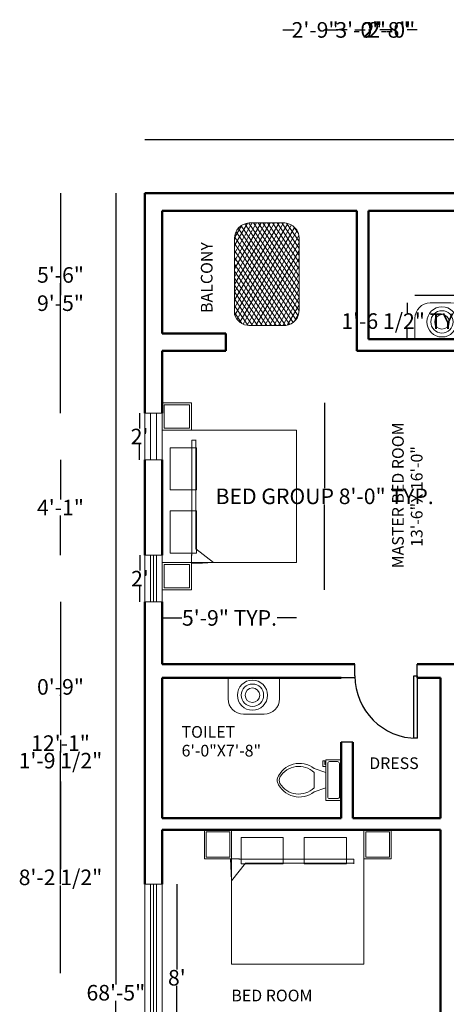
# Model space of a CAD drawing. Units: inches. Extents: x -135167 to -134597, y 156853 to 157819.
# Tile 3 of 5: x -135167 to -134948, y 157306 to 157812. Entities that reach past the tile are written whole.
import ezdxf

# ---------------------------------------------------------------- set-up
doc = ezdxf.new("R2010")
doc.units = ezdxf.units.IN
doc.header["$MEASUREMENT"] = 0
for name, color, linetype, lineweight in [('A-ANNO-DIMS', 4, 'Continuous', 18), ('A-AREA-IDEN', 76, 'Continuous', 25), ('A-FLOR-FIXT', 3, 'Continuous', 20), ('A-FLOR-PATT', 8, 'Continuous', 13), ('A-FURN', 1, 'Continuous', 18), ('doors', 5, 'Continuous', 25), ('walls', 2, 'Continuous', 50), ('window', 6, 'Continuous', 18)]:
    doc.layers.add(name, color=color, linetype=linetype, lineweight=lineweight)
doc.styles.get("Standard").update_dxf_attribs({"font": 'arial.ttf'})
doc.dimstyles.get("Standard").update_dxf_attribs({"dimtxt": 8, "dimasz": 0.18, "dimexe": 0.18, "dimexo": 0.0625, "dimgap": 0.09, "dimtad": 0, "dimtih": 1, "dimtoh": 1, "dimdec": 0, "dimzin": 0, "dimdsep": 46, "dimlunit": 3, "dimtxsty": 'Standard', "dimblk": 'ARCHTICK', "dimcen": 0.09, "dimse1": 1, "dimse2": 1, "dimadec": 0, "dimazin": 0, "dimtfac": 1, "dimtdec": 0, "dimtofl": 0, "dimtmove": 0, "dimatfit": 3, "dimldrblk": 'DOTSMALL', "dimfxl": 1, "dimtolj": 1, "dimtzin": 0, "dimarcsym": 0})

# ---------------------------------------------------------------- blocks, each defined once
blk = doc.blocks.new('*U11')
for p, q in [((-32, 0), (-32, 6)), ((0, 0), (0, 6))]:
    blk.add_line(p, q)
blk.add_lwpolyline([(0, 0), (0, -32), (-1.75, -32), (-1.75, 0)], close=True)
blk.add_arc((0, 0), 32, 180, 270)
blk = doc.blocks.new('*U16')
for p, q in [((-8.01, 3.98), (-14.01, 5.97)), ((-9.51, 6.98), (-9.52, 9.98)), ((-9.52, 9.98), (-8.52, 9.98)), ((-8.01, 6.98), (-9.51, 6.98)), ((-8.52, 9.98), (-8.52, 7.98)), ((-8.52, 7.98), (-8.02, 7.98)), ((-13.99, -4.03), (-14.01, 3.97)), ((-7.99, -4.02), (-13.99, -6.03)), ((-5.98, -9.51), (-1.98, -9.5))]:
    blk.add_line(p, q)
blk.add_lwpolyline([(-7.98, -10.51), (0.02, -10.5), (-0.02, 10.5), (-8.02, 10.48)], close=True)
for points in [[(-7.02, 8.49), (-6.98, -8.51)], [(-2.02, 9.5), (-6.02, 9.49)], [(-0.98, -8.5), (-1.02, 8.5)]]:
    blk.add_lwpolyline(points)
for centre, radius, start, end in [((-21.57, -3.56), 12.17, 51.5766, 158.079), ((-21.81, -4.24), 11.33, 46.4753, 149.0544), ((-6.14, 8.61), 0.884, 81.9774, 188.2376), ((-1.89, 8.62), 0.884, 351.9774, 98.2376), ((-29, -0.05), 4, 164.9681, 195.247), ((-27.88, -0.05), 4, 155.8394, 204.3757), ((-21.59, 3.48), 12.17, 202.136, 308.6382), ((-21.83, 4.16), 11.33, 211.1605, 313.7396), ((-6.11, -8.64), 0.884, 171.9774, 278.2376), ((-1.86, -8.63), 0.884, 261.9774, 8.2376)]:
    blk.add_arc(centre, radius, start, end)
blk = doc.blocks.new('_ArchTick')
at = {"color": 0, "linetype": 'ByBlock', "const_width": 0.15}
blk.add_lwpolyline([(-0.5, -0.5), (0.5, 0.5)], dxfattribs=at)
blk = doc.blocks.new('*D19')
at = {"layer": 'A-ANNO-DIMS', "color": 0, "lineweight": -2, "transparency": 16777216}
for p, q in [((-135102.89, 157750.46), (-134940.89, 157750.46)), ((-134744.89, 157750.46), (-134906.88, 157750.46))]:
    blk.add_line(p, q, dxfattribs=at)
at = {"layer": 'Defpoints', "color": 0, "transparency": 16777216}
for p in [(-134744.89, 157750.46), (-135102.89, 157722.94), (-134744.89, 157722.94)]:
    blk.add_point(p, dxfattribs=at)
at = {"layer": 'A-ANNO-DIMS', "color": 0, "lineweight": -2, "transparency": 16777216, "xscale": 0.18, "yscale": 0.18, "zscale": 0.18, "rotation": 180}
blk.add_blockref('_ArchTick', (-135102.89, 157750.46), dxfattribs=at)
at = {"layer": 'A-ANNO-DIMS', "color": 0, "lineweight": -2, "transparency": 16777216, "xscale": 0.18, "yscale": 0.18, "zscale": 0.18}
blk.add_blockref('_ArchTick', (-134744.89, 157750.46), dxfattribs=at)
at = {"layer": 'A-ANNO-DIMS', "color": 0, "transparency": 16777216, "insert": (-134923.89, 157750.46), "char_height": 8, "attachment_point": 5}
blk.add_mtext('\\A1;29\'-10"', dxfattribs=at)
blk = doc.blocks.new('_DotSmall')
at = {"color": 0, "linetype": 'ByBlock', "const_width": 0.5}
blk.add_lwpolyline([(-0.0625, 0, 1), (0.0625, 0, 1)], format="xyb", close=True, dxfattribs=at)
blk = doc.blocks.new('*D20')
at = {"layer": 'A-ANNO-DIMS', "color": 0, "lineweight": -2, "transparency": 16777216}
for p, q in [((-135117.79, 157722.94), (-135117.79, 157316.42)), ((-135117.79, 156901.55), (-135117.79, 157308.07))]:
    blk.add_line(p, q, dxfattribs=at)
at = {"layer": 'Defpoints', "color": 0, "transparency": 16777216}
for p in [(-135117.79, 157722.94), (-135102.89, 157722.94), (-135102.89, 156901.55)]:
    blk.add_point(p, dxfattribs=at)
at = {"layer": 'A-ANNO-DIMS', "color": 0, "lineweight": -2, "transparency": 16777216, "xscale": 0.18, "yscale": 0.18, "zscale": 0.18}
for p, rotation in [((-135117.79, 157722.94), 90), ((-135117.79, 156901.55), 270)]:
    blk.add_blockref('_ArchTick', p, dxfattribs=dict(at, rotation=rotation))
at = {"layer": 'A-ANNO-DIMS', "color": 0, "transparency": 16777216, "insert": (-135117.79, 157312.25), "char_height": 8, "attachment_point": 5}
blk.add_mtext('\\A1;68\'-5"', dxfattribs=at)
blk = doc.blocks.new('*D31')
at = {"layer": 'A-ANNO-DIMS', "color": 0, "lineweight": -2, "transparency": 16777216}
for p, q in [((-135105.6, 157609.94), (-135105.6, 157602.05)), ((-135105.6, 157585.94), (-135105.6, 157593.84))]:
    blk.add_line(p, q, dxfattribs=at)
at = {"layer": 'Defpoints', "color": 0, "transparency": 16777216}
for p in [(-135102.89, 157609.94), (-135105.6, 157585.94), (-135102.89, 157585.94)]:
    blk.add_point(p, dxfattribs=at)
at = {"layer": 'A-ANNO-DIMS', "color": 0, "lineweight": -2, "transparency": 16777216, "xscale": 0.18, "yscale": 0.18, "zscale": 0.18}
for p, rotation in [((-135105.6, 157609.94), 90), ((-135105.6, 157585.94), 270)]:
    blk.add_blockref('_ArchTick', p, dxfattribs=dict(at, rotation=rotation))
at = {"layer": 'A-ANNO-DIMS', "color": 0, "transparency": 16777216, "insert": (-135105.6, 157597.94), "char_height": 8, "attachment_point": 5}
blk.add_mtext("\\A1;2'", dxfattribs=at)
blk = doc.blocks.new('*D32')
at = {"layer": 'A-ANNO-DIMS', "color": 0, "lineweight": -2, "transparency": 16777216}
for p, q in [((-135105.42, 157536.94), (-135105.42, 157529.05)), ((-135105.42, 157512.94), (-135105.42, 157520.84))]:
    blk.add_line(p, q, dxfattribs=at)
at = {"layer": 'Defpoints', "color": 0, "transparency": 16777216}
for p in [(-135102.89, 157536.94), (-135105.42, 157512.94), (-135102.89, 157512.94)]:
    blk.add_point(p, dxfattribs=at)
at = {"layer": 'A-ANNO-DIMS', "color": 0, "lineweight": -2, "transparency": 16777216, "xscale": 0.18, "yscale": 0.18, "zscale": 0.18}
for p, rotation in [((-135105.42, 157536.94), 90), ((-135105.42, 157512.94), 270)]:
    blk.add_blockref('_ArchTick', p, dxfattribs=dict(at, rotation=rotation))
at = {"layer": 'A-ANNO-DIMS', "color": 0, "transparency": 16777216, "insert": (-135105.42, 157524.94), "char_height": 8, "attachment_point": 5}
blk.add_mtext("\\A1;2'", dxfattribs=at)
blk = doc.blocks.new('*D33')
at = {"layer": 'A-ANNO-DIMS', "color": 0, "lineweight": -2, "transparency": 16777216}
for p, q in [((-135086.43, 157367.94), (-135086.43, 157324.12)), ((-135086.43, 157271.94), (-135086.43, 157315.77))]:
    blk.add_line(p, q, dxfattribs=at)
at = {"layer": 'Defpoints', "color": 0, "transparency": 16777216}
for p in [(-135093.89, 157367.94), (-135086.43, 157367.94), (-135093.89, 157271.94)]:
    blk.add_point(p, dxfattribs=at)
at = {"layer": 'A-ANNO-DIMS', "color": 0, "lineweight": -2, "transparency": 16777216, "xscale": 0.18, "yscale": 0.18, "zscale": 0.18}
for p, rotation in [((-135086.43, 157367.94), 90), ((-135086.43, 157271.94), 270)]:
    blk.add_blockref('_ArchTick', p, dxfattribs=dict(at, rotation=rotation))
at = {"layer": 'A-ANNO-DIMS', "color": 0, "transparency": 16777216, "insert": (-135086.43, 157319.94), "char_height": 8, "attachment_point": 5}
blk.add_mtext("\\A1;8'", dxfattribs=at)
blk = doc.blocks.new('BED-DOUBLE-WITH-NIGHTSTANDS')
for p, q in [((0, 82.04), (69, 82.04)), ((69, 82.04), (69, 14.04)), ((15.15, 17.72), (15.15, 76.81)), ((15.15, 76.81), (17.47, 76.81)), ((17.23, 76.81), (17.23, 21.1)), ((17.23, 21.1), (26.3, 14.04)), ((15.01, 13.43), (15.01, 18.09)), ((69, 14.04), (0, 14.04)), ((26.3, 14.04), (15.01, 13.43))]:
    blk.add_line(p, q)
for points in [[(0, 96.09), (15.01, 96.09), (15.01, 82.04), (0, 82.04)], [(1, 95.09), (14.01, 95.09), (14.01, 83.04), (1, 83.04)], [(3.95, 51.37), (17.49, 51.37), (17.49, 73.01), (3.95, 73.01)], [(3.95, 18.92), (17.49, 18.92), (17.49, 40.56), (3.95, 40.56)], [(0, 14.04), (15.01, 14.04), (15.01, 0), (0, 0)], [(1, 13.04), (14.01, 13.04), (14.01, 1), (1, 1)]]:
    blk.add_lwpolyline(points, close=True)
blk = doc.blocks.new('BASIN-WALL')
for points in [[(18.54, 18.59), (7.9, 18.59)], [(0, 10.69), (0, 0)], [(26.44, 0), (26.44, 10.69)]]:
    blk.add_lwpolyline(points)
for radius in [7.75, 5.75, 3.75]:
    blk.add_circle((13.93, 8.88), radius)
for centre, start, end in [((7.9, 10.69), 90, 180), ((18.54, 10.69), 0, 90)]:
    blk.add_arc(centre, 7.9, start, end)
blk = doc.blocks.new('WIN-96IN')
for p, q in [((0, 96), (9, 96)), ((0, 96), (0, 0)), ((3, 96), (3, 0)), ((4.5, 96), (4.5, 0)), ((6, 96), (6, 0)), ((9, 96), (9, 0)), ((0, 0), (9, 0))]:
    blk.add_line(p, q)
blk = doc.blocks.new('WIN-24IN')
for p, q in [((0, 24), (9, 24)), ((0, 24), (0, 0)), ((3, 24), (3, 0)), ((4.5, 24), (4.5, 0)), ((6, 24), (6, 0)), ((9, 24), (9, 0)), ((0, 0), (9, 0))]:
    blk.add_line(p, q)
blk = doc.blocks.new('*D48')
at = {"layer": 'A-ANNO-DIMS', "color": 0, "lineweight": -2, "transparency": 16777216}
for p, q in [((-135010.47, 157615.27), (-135010.47, 157571.45)), ((-135010.47, 157519.18), (-135010.47, 157562.99))]:
    blk.add_line(p, q, dxfattribs=at)
at = {"layer": 'Defpoints', "color": 0, "transparency": 16777216}
for p in [(-135024.89, 157615.27), (-135010.47, 157615.27), (-135024.89, 157519.18)]:
    blk.add_point(p, dxfattribs=at)
at = {"layer": 'A-ANNO-DIMS', "color": 0, "lineweight": -2, "transparency": 16777216, "xscale": 0.18, "yscale": 0.18, "zscale": 0.18}
for p, rotation in [((-135010.47, 157615.27), 90), ((-135010.47, 157519.18), 270)]:
    blk.add_blockref('_ArchTick', p, dxfattribs=dict(at, rotation=rotation))
at = {"layer": 'A-ANNO-DIMS', "color": 0, "transparency": 16777216, "insert": (-135010.47, 157567.22), "char_height": 8, "attachment_point": 5}
blk.add_mtext('\\A1;BED GROUP 8\'-0" TYP.', dxfattribs=at)
blk = doc.blocks.new('*D49')
at = {"layer": 'A-ANNO-DIMS', "color": 0, "lineweight": -2, "transparency": 16777216}
for p, q in [((-135093.89, 157504.77), (-135083.86, 157504.77)), ((-135024.89, 157504.77), (-135034.91, 157504.77))]:
    blk.add_line(p, q, dxfattribs=at)
at = {"layer": 'Defpoints', "color": 0, "transparency": 16777216}
for p in [(-135093.89, 157519.18), (-135024.89, 157519.18), (-135024.89, 157504.77)]:
    blk.add_point(p, dxfattribs=at)
at = {"layer": 'A-ANNO-DIMS', "color": 0, "lineweight": -2, "transparency": 16777216, "xscale": 0.18, "yscale": 0.18, "zscale": 0.18, "rotation": 180}
blk.add_blockref('_ArchTick', (-135093.89, 157504.77), dxfattribs=at)
at = {"layer": 'A-ANNO-DIMS', "color": 0, "lineweight": -2, "transparency": 16777216, "xscale": 0.18, "yscale": 0.18, "zscale": 0.18}
blk.add_blockref('_ArchTick', (-135024.89, 157504.77), dxfattribs=at)
at = {"layer": 'A-ANNO-DIMS', "color": 0, "transparency": 16777216, "insert": (-135059.39, 157504.77), "char_height": 8, "attachment_point": 5}
blk.add_mtext('\\A1;5\'-9" TYP.', dxfattribs=at)
blk = doc.blocks.new('*D52')
at = {"layer": 'A-ANNO-DIMS', "color": 0, "lineweight": -2, "transparency": 16777216}
for p, q in [((-134964.09, 157670.5), (-134937.65, 157670.5)), ((-134937.65, 157670.5), (-134937.47, 157670.5))]:
    blk.add_line(p, q, dxfattribs=at)
at = {"layer": 'Defpoints', "color": 0, "transparency": 16777216}
for p in [(-134964.09, 157666.53), (-134937.65, 157670.5), (-134937.65, 157666.53)]:
    blk.add_point(p, dxfattribs=at)
at = {"layer": 'A-ANNO-DIMS', "color": 0, "lineweight": -2, "transparency": 16777216, "xscale": 0.18, "yscale": 0.18, "zscale": 0.18, "rotation": 180}
blk.add_blockref('_ArchTick', (-134964.09, 157670.5), dxfattribs=at)
at = {"layer": 'A-ANNO-DIMS', "color": 0, "lineweight": -2, "transparency": 16777216, "xscale": 0.18, "yscale": 0.18, "zscale": 0.18}
blk.add_blockref('_ArchTick', (-134937.65, 157670.5), dxfattribs=at)
at = {"layer": 'A-ANNO-DIMS', "color": 0, "transparency": 16777216, "insert": (-134885.53, 157670.5), "char_height": 8, "attachment_point": 5}
blk.add_mtext('\\A1;BASIN 2\'-2 1/2" TYP.', dxfattribs=at)
blk = doc.blocks.new('*D53')
at = {"layer": 'A-ANNO-DIMS', "color": 0, "lineweight": -2, "transparency": 16777216}
for p, q in [((-134968.06, 157666.53), (-134968.06, 157661.46)), ((-134968.06, 157647.94), (-134968.06, 157653.01))]:
    blk.add_line(p, q, dxfattribs=at)
at = {"layer": 'Defpoints', "color": 0, "transparency": 16777216}
for p in [(-134968.06, 157666.53), (-134964.09, 157666.53), (-134964.09, 157647.94)]:
    blk.add_point(p, dxfattribs=at)
at = {"layer": 'A-ANNO-DIMS', "color": 0, "lineweight": -2, "transparency": 16777216, "xscale": 0.18, "yscale": 0.18, "zscale": 0.18}
for p, rotation in [((-134968.06, 157666.53), 90), ((-134968.06, 157647.94), 270)]:
    blk.add_blockref('_ArchTick', p, dxfattribs=dict(at, rotation=rotation))
at = {"layer": 'A-ANNO-DIMS', "color": 0, "transparency": 16777216, "insert": (-134968.06, 157657.24), "char_height": 8, "attachment_point": 5}
blk.add_mtext('\\A1;1\'-6 1/2" TYP.', dxfattribs=at)
blk = doc.blocks.new('*D56')
at = {"layer": 'A-ANNO-DIMS', "color": 0, "lineweight": -2, "transparency": 16777216}
for p, q in [((-135146.24, 157722.94), (-135146.24, 157670.62)), ((-135146.24, 157609.94), (-135146.24, 157662.27))]:
    blk.add_line(p, q, dxfattribs=at)
at = {"layer": 'Defpoints', "color": 0, "transparency": 16777216}
for p in [(-135102.89, 157722.94), (-135146.24, 157609.94), (-135102.89, 157609.94)]:
    blk.add_point(p, dxfattribs=at)
at = {"layer": 'A-ANNO-DIMS', "color": 0, "lineweight": -2, "transparency": 16777216, "xscale": 0.18, "yscale": 0.18, "zscale": 0.18}
for p, rotation in [((-135146.24, 157722.94), 90), ((-135146.24, 157609.94), 270)]:
    blk.add_blockref('_ArchTick', p, dxfattribs=dict(at, rotation=rotation))
at = {"layer": 'A-ANNO-DIMS', "color": 0, "transparency": 16777216, "insert": (-135146.24, 157666.44), "char_height": 8, "attachment_point": 5}
blk.add_mtext('\\A1;9\'-5"', dxfattribs=at)
blk = doc.blocks.new('*D57')
at = {"layer": 'A-ANNO-DIMS', "color": 0, "lineweight": -2, "transparency": 16777216}
for p, q in [((-135146.24, 157585.94), (-135146.24, 157565.55)), ((-135146.24, 157536.94), (-135146.24, 157557.34))]:
    blk.add_line(p, q, dxfattribs=at)
at = {"layer": 'Defpoints', "color": 0, "transparency": 16777216}
for p in [(-135102.89, 157585.94), (-135146.24, 157536.94), (-135102.89, 157536.94)]:
    blk.add_point(p, dxfattribs=at)
at = {"layer": 'A-ANNO-DIMS', "color": 0, "lineweight": -2, "transparency": 16777216, "xscale": 0.18, "yscale": 0.18, "zscale": 0.18}
for p, rotation in [((-135146.24, 157585.94), 90), ((-135146.24, 157536.94), 270)]:
    blk.add_blockref('_ArchTick', p, dxfattribs=dict(at, rotation=rotation))
at = {"layer": 'A-ANNO-DIMS', "color": 0, "transparency": 16777216, "insert": (-135146.24, 157561.44), "char_height": 8, "attachment_point": 5}
blk.add_mtext('\\A1;4\'-1"', dxfattribs=at)
blk = doc.blocks.new('*D58')
at = {"layer": 'A-ANNO-DIMS', "color": 0, "lineweight": -2, "transparency": 16777216}
for p, q in [((-135146.24, 157512.94), (-135146.24, 157444.55)), ((-135146.24, 157367.94), (-135146.24, 157436.34))]:
    blk.add_line(p, q, dxfattribs=at)
at = {"layer": 'Defpoints', "color": 0, "transparency": 16777216}
for p in [(-135102.89, 157512.94), (-135146.24, 157367.94), (-135102.89, 157367.94)]:
    blk.add_point(p, dxfattribs=at)
at = {"layer": 'A-ANNO-DIMS', "color": 0, "lineweight": -2, "transparency": 16777216, "xscale": 0.18, "yscale": 0.18, "zscale": 0.18}
for p, rotation in [((-135146.24, 157512.94), 90), ((-135146.24, 157367.94), 270)]:
    blk.add_blockref('_ArchTick', p, dxfattribs=dict(at, rotation=rotation))
at = {"layer": 'A-ANNO-DIMS', "color": 0, "transparency": 16777216, "insert": (-135146.24, 157440.44), "char_height": 8, "attachment_point": 5}
blk.add_mtext('\\A1;12\'-1"', dxfattribs=at)
blk = doc.blocks.new('*D74')
at = {"layer": 'A-ANNO-DIMS', "color": 0, "lineweight": -2, "transparency": 16777216}
for p, q in [((-135146.24, 157420.8), (-135146.24, 157375.74)), ((-135146.24, 157322.23), (-135146.24, 157367.29))]:
    blk.add_line(p, q, dxfattribs=at)
at = {"layer": 'Defpoints', "color": 0, "transparency": 16777216}
for p in [(-134842.49, 157420.8), (-135146.24, 157322.23), (-134842.49, 157322.23)]:
    blk.add_point(p, dxfattribs=at)
at = {"layer": 'A-ANNO-DIMS', "color": 0, "lineweight": -2, "transparency": 16777216, "xscale": 0.18, "yscale": 0.18, "zscale": 0.18}
for p, rotation in [((-135146.24, 157420.8), 90), ((-135146.24, 157322.23), 270)]:
    blk.add_blockref('_ArchTick', p, dxfattribs=dict(at, rotation=rotation))
at = {"layer": 'A-ANNO-DIMS', "color": 0, "transparency": 16777216, "insert": (-135146.24, 157371.51), "char_height": 8, "attachment_point": 5}
blk.add_mtext('\\A1;8\'-2 1/2"', dxfattribs=at)
blk = doc.blocks.new('*D75')
at = {"layer": 'A-ANNO-DIMS', "color": 0, "lineweight": -2, "transparency": 16777216}
for p, q in [((-135146.24, 157473.94), (-135146.24, 157473.51)), ((-135146.24, 157464.74), (-135146.24, 157465.17))]:
    blk.add_line(p, q, dxfattribs=at)
at = {"layer": 'Defpoints', "color": 0, "transparency": 16777216}
for p in [(-135146.24, 157473.94), (-134849.54, 157473.94), (-134848.8, 157464.74)]:
    blk.add_point(p, dxfattribs=at)
at = {"layer": 'A-ANNO-DIMS', "color": 0, "lineweight": -2, "transparency": 16777216, "xscale": 0.18, "yscale": 0.18, "zscale": 0.18}
for p, rotation in [((-135146.24, 157473.94), 90), ((-135146.24, 157464.74), 270)]:
    blk.add_blockref('_ArchTick', p, dxfattribs=dict(at, rotation=rotation))
at = {"layer": 'A-ANNO-DIMS', "color": 0, "transparency": 16777216, "insert": (-135146.24, 157469.34), "char_height": 8, "attachment_point": 5}
blk.add_mtext('\\A1;0\'-9"', dxfattribs=at)
blk = doc.blocks.new('*D78')
at = {"layer": 'A-ANNO-DIMS', "color": 0, "lineweight": -2, "transparency": 16777216}
for p, q in [((-135146.24, 157442.1), (-135146.24, 157435.68)), ((-135146.24, 157420.8), (-135146.24, 157427.22))]:
    blk.add_line(p, q, dxfattribs=at)
at = {"layer": 'Defpoints', "color": 0, "transparency": 16777216}
for p in [(-135146.24, 157442.1), (-134848.8, 157442.1), (-134842.49, 157420.8)]:
    blk.add_point(p, dxfattribs=at)
at = {"layer": 'A-ANNO-DIMS', "color": 0, "lineweight": -2, "transparency": 16777216, "xscale": 0.18, "yscale": 0.18, "zscale": 0.18}
for p, rotation in [((-135146.24, 157442.1), 90), ((-135146.24, 157420.8), 270)]:
    blk.add_blockref('_ArchTick', p, dxfattribs=dict(at, rotation=rotation))
at = {"layer": 'A-ANNO-DIMS', "color": 0, "transparency": 16777216, "insert": (-135146.24, 157431.45), "char_height": 8, "attachment_point": 5}
blk.add_mtext('\\A1;1\'-9 1/2"', dxfattribs=at)
blk = doc.blocks.new('*D83')
at = {"layer": 'A-ANNO-DIMS', "color": 0, "lineweight": -2, "transparency": 16777216}
for p, q in [((-134994.89, 157806.8), (-134989.68, 157806.8)), ((-134962.89, 157806.8), (-134968.09, 157806.8))]:
    blk.add_line(p, q, dxfattribs=at)
at = {"layer": 'Defpoints', "color": 0, "transparency": 16777216}
for p in [(-134962.89, 157806.8), (-134994.89, 157480.94), (-134962.89, 157480.94)]:
    blk.add_point(p, dxfattribs=at)
at = {"layer": 'A-ANNO-DIMS', "color": 0, "lineweight": -2, "transparency": 16777216, "xscale": 0.18, "yscale": 0.18, "zscale": 0.18, "rotation": 180}
blk.add_blockref('_ArchTick', (-134994.89, 157806.8), dxfattribs=at)
at = {"layer": 'A-ANNO-DIMS', "color": 0, "lineweight": -2, "transparency": 16777216, "xscale": 0.18, "yscale": 0.18, "zscale": 0.18}
blk.add_blockref('_ArchTick', (-134962.89, 157806.8), dxfattribs=at)
at = {"layer": 'A-ANNO-DIMS', "color": 0, "transparency": 16777216, "insert": (-134978.89, 157806.8), "char_height": 8, "attachment_point": 5}
blk.add_mtext('\\A1;2\'-8"', dxfattribs=at)
blk = doc.blocks.new('*D86')
at = {"layer": 'A-ANNO-DIMS', "color": 0, "lineweight": -2, "transparency": 16777216}
for p, q in [((-135010.89, 157806.8), (-135003.61, 157806.8)), ((-134974.89, 157806.8), (-134982.17, 157806.8))]:
    blk.add_line(p, q, dxfattribs=at)
at = {"layer": 'Defpoints', "color": 0, "transparency": 16777216}
for p in [(-134974.89, 157806.8), (-135010.89, 157117.94), (-134974.89, 157117.94)]:
    blk.add_point(p, dxfattribs=at)
at = {"layer": 'A-ANNO-DIMS', "color": 0, "lineweight": -2, "transparency": 16777216, "xscale": 0.18, "yscale": 0.18, "zscale": 0.18, "rotation": 180}
blk.add_blockref('_ArchTick', (-135010.89, 157806.8), dxfattribs=at)
at = {"layer": 'A-ANNO-DIMS', "color": 0, "lineweight": -2, "transparency": 16777216, "xscale": 0.18, "yscale": 0.18, "zscale": 0.18}
blk.add_blockref('_ArchTick', (-134974.89, 157806.8), dxfattribs=at)
at = {"layer": 'A-ANNO-DIMS', "color": 0, "transparency": 16777216, "insert": (-134992.89, 157806.8), "char_height": 8, "attachment_point": 5}
blk.add_mtext('\\A1;3\'-0"', dxfattribs=at)
blk = doc.blocks.new('*D88')
at = {"layer": 'A-ANNO-DIMS', "color": 0, "lineweight": -2, "transparency": 16777216}
for p, q in [((-135031.89, 157806.8), (-135026.18, 157806.8)), ((-134998.89, 157806.8), (-135004.59, 157806.8))]:
    blk.add_line(p, q, dxfattribs=at)
at = {"layer": 'Defpoints', "color": 0, "transparency": 16777216}
for p in [(-134998.89, 157806.8), (-135031.89, 156966.94), (-134998.89, 156966.94)]:
    blk.add_point(p, dxfattribs=at)
at = {"layer": 'A-ANNO-DIMS', "color": 0, "lineweight": -2, "transparency": 16777216, "xscale": 0.18, "yscale": 0.18, "zscale": 0.18, "rotation": 180}
blk.add_blockref('_ArchTick', (-135031.89, 157806.8), dxfattribs=at)
at = {"layer": 'A-ANNO-DIMS', "color": 0, "lineweight": -2, "transparency": 16777216, "xscale": 0.18, "yscale": 0.18, "zscale": 0.18}
blk.add_blockref('_ArchTick', (-134998.89, 157806.8), dxfattribs=at)
at = {"layer": 'A-ANNO-DIMS', "color": 0, "transparency": 16777216, "insert": (-135015.39, 157806.8), "char_height": 8, "attachment_point": 5}
blk.add_mtext('\\A1;2\'-9"', dxfattribs=at)
blk = doc.blocks.new('*D92')
at = {"layer": 'A-ANNO-DIMS', "color": 0, "lineweight": -2, "transparency": 16777216}
for p, q in [((-134987.89, 156858.2), (-134955.58, 156858.2)), ((-134901.89, 156858.2), (-134934.2, 156858.2))]:
    blk.add_line(p, q, dxfattribs=at)
at = {"layer": 'Defpoints', "color": 0, "transparency": 16777216}
for p in [(-134987.89, 157647.94), (-134901.89, 157647.94), (-134901.89, 156858.2)]:
    blk.add_point(p, dxfattribs=at)
at = {"layer": 'A-ANNO-DIMS', "color": 0, "lineweight": -2, "transparency": 16777216, "xscale": 0.18, "yscale": 0.18, "zscale": 0.18, "rotation": 180}
blk.add_blockref('_ArchTick', (-134987.89, 156858.2), dxfattribs=at)
at = {"layer": 'A-ANNO-DIMS', "color": 0, "lineweight": -2, "transparency": 16777216, "xscale": 0.18, "yscale": 0.18, "zscale": 0.18}
blk.add_blockref('_ArchTick', (-134901.89, 156858.2), dxfattribs=at)
at = {"layer": 'A-ANNO-DIMS', "color": 0, "transparency": 16777216, "insert": (-134944.89, 156858.2), "char_height": 8, "attachment_point": 5}
blk.add_mtext('\\A1;7\'-2"', dxfattribs=at)
blk = doc.blocks.new('*D93')
at = {"layer": 'A-ANNO-DIMS', "color": 0, "lineweight": -2, "transparency": 16777216}
for p, q in [((-135146.24, 157713.94), (-135146.24, 157685.12)), ((-135146.24, 157647.94), (-135146.24, 157676.77))]:
    blk.add_line(p, q, dxfattribs=at)
at = {"layer": 'Defpoints', "color": 0, "transparency": 16777216}
for p in [(-134987.89, 157713.94), (-135146.24, 157647.94), (-134987.89, 157647.94)]:
    blk.add_point(p, dxfattribs=at)
at = {"layer": 'A-ANNO-DIMS', "color": 0, "lineweight": -2, "transparency": 16777216, "xscale": 0.18, "yscale": 0.18, "zscale": 0.18}
for p, rotation in [((-135146.24, 157713.94), 90), ((-135146.24, 157647.94), 270)]:
    blk.add_blockref('_ArchTick', p, dxfattribs=dict(at, rotation=rotation))
at = {"layer": 'A-ANNO-DIMS', "color": 0, "transparency": 16777216, "insert": (-135146.24, 157680.94), "char_height": 8, "attachment_point": 5}
blk.add_mtext('\\A1;5\'-6"', dxfattribs=at)
blk = doc.blocks.new('*D94')
at = {"layer": 'A-ANNO-DIMS', "color": 0, "lineweight": -2, "transparency": 16777216}
for p, q in [((-134987.89, 157806.8), (-134986.78, 157806.8)), ((-134964.09, 157806.8), (-134965.2, 157806.8))]:
    blk.add_line(p, q, dxfattribs=at)
at = {"layer": 'Defpoints', "color": 0, "transparency": 16777216}
for p in [(-134964.09, 157806.8), (-134987.89, 157647.94), (-134964.09, 157647.94)]:
    blk.add_point(p, dxfattribs=at)
at = {"layer": 'A-ANNO-DIMS', "color": 0, "lineweight": -2, "transparency": 16777216, "xscale": 0.18, "yscale": 0.18, "zscale": 0.18, "rotation": 180}
blk.add_blockref('_ArchTick', (-134987.89, 157806.8), dxfattribs=at)
at = {"layer": 'A-ANNO-DIMS', "color": 0, "lineweight": -2, "transparency": 16777216, "xscale": 0.18, "yscale": 0.18, "zscale": 0.18}
blk.add_blockref('_ArchTick', (-134964.09, 157806.8), dxfattribs=at)
at = {"layer": 'A-ANNO-DIMS', "color": 0, "transparency": 16777216, "insert": (-134975.99, 157806.8), "char_height": 8, "attachment_point": 5}
blk.add_mtext('\\A1;2\'-0"', dxfattribs=at)

msp = doc.modelspace()

# ---------------------------------------------------------------- hatches: boundary and pattern name
at = {"layer": 'A-FLOR-PATT'}
h = msp.add_hatch(dxfattribs=at)
h.set_pattern_fill('ANSI31', color=256, scale=16, angle=14.987203, style=0)
h.paths.add_polyline_path([(-135030.49, 157655.04), (-135029.55, 157655.21), (-135028.63, 157655.49), (-135027.76, 157655.89), (-135026.94, 157656.38), (-135026.18, 157656.98), (-135025.5, 157657.66), (-135024.91, 157658.42), (-135024.42, 157659.24), (-135024.03, 157660.12), (-135023.75, 157661.03), (-135023.58, 157661.98), (-135023.53, 157662.94), (-135023.53, 157699.8), (-135023.59, 157700.71), (-135023.76, 157701.61), (-135024.02, 157702.49), (-135024.39, 157703.33), (-135024.86, 157704.12), (-135025.41, 157704.85), (-135026.04, 157705.51), (-135026.74, 157706.1), (-135027.51, 157706.6), (-135028.33, 157707), (-135029.19, 157707.31), (-135030.09, 157707.52), (-135031, 157707.62), (-135049.3, 157707.62), (-135050.24, 157707.52), (-135051.15, 157707.3), (-135052.03, 157706.97), (-135052.87, 157706.55), (-135053.65, 157706.02), (-135054.37, 157705.41), (-135055, 157704.71), (-135055.55, 157703.95), (-135056, 157703.12), (-135056.35, 157702.25), (-135056.6, 157701.34), (-135056.74, 157700.41), (-135056.76, 157699.47), (-135056.76, 157660.62), (-135056.43, 157659.75), (-135056.01, 157658.92), (-135055.49, 157658.15), (-135054.88, 157657.44), (-135054.19, 157656.81), (-135053.44, 157656.26), (-135052.62, 157655.81), (-135051.76, 157655.46), (-135050.86, 157655.21), (-135049.94, 157655.07), (-135049.01, 157655.04)])
h = msp.add_hatch(dxfattribs=at)
h.set_pattern_fill('ANSI31', color=256, scale=16, angle=79.3093735, style=0)
h.paths.add_polyline_path([(-135030.49, 157655.04), (-135029.55, 157655.21), (-135028.63, 157655.49), (-135027.76, 157655.89), (-135026.94, 157656.38), (-135026.18, 157656.98), (-135025.5, 157657.66), (-135024.91, 157658.42), (-135024.42, 157659.24), (-135024.03, 157660.12), (-135023.75, 157661.03), (-135023.58, 157661.98), (-135023.53, 157662.94), (-135023.53, 157699.8), (-135023.59, 157700.71), (-135023.76, 157701.61), (-135024.02, 157702.49), (-135024.39, 157703.33), (-135024.86, 157704.12), (-135025.41, 157704.85), (-135026.04, 157705.51), (-135026.74, 157706.1), (-135027.51, 157706.6), (-135028.33, 157707), (-135029.19, 157707.31), (-135030.09, 157707.52), (-135031, 157707.62), (-135049.3, 157707.62), (-135050.24, 157707.52), (-135051.15, 157707.3), (-135052.03, 157706.97), (-135052.87, 157706.55), (-135053.65, 157706.02), (-135054.37, 157705.41), (-135055, 157704.71), (-135055.55, 157703.95), (-135056, 157703.12), (-135056.35, 157702.25), (-135056.6, 157701.34), (-135056.74, 157700.41), (-135056.76, 157699.47), (-135056.76, 157660.62), (-135056.43, 157659.75), (-135056.01, 157658.92), (-135055.49, 157658.15), (-135054.88, 157657.44), (-135054.19, 157656.81), (-135053.44, 157656.26), (-135052.62, 157655.81), (-135051.76, 157655.46), (-135050.86, 157655.21), (-135049.94, 157655.07), (-135049.01, 157655.04)])

# ---------------------------------------------------------------- linework, layer by layer
at = {"layer": 'A-FURN'}
for points in [[(-135049.3, 157707.62), (-135031, 157707.62)], [(-135056.76, 157660.62), (-135056.76, 157700.01)], [(-135023.53, 157699.8), (-135023.53, 157662.82)], [(-135030.49, 157655.04), (-135049.41, 157655.04)]]:
    msp.add_lwpolyline(points, dxfattribs=at)
for centre, start, end in [((-135048.87, 157699.74), 93.1432, 181.9421), ((-135031.43, 157699.74), 0.4238, 86.8568), ((-135031.43, 157662.88), 276.7927, 0.4238), ((-135049.21, 157662.93), 197.0139, 271.4589)]:
    msp.add_arc(centre, 7.9, start, end, dxfattribs=at)
at = {"layer": 'doors'}
for p, q in [((-134962.89, 157473.94), (-134962.89, 157480.94)), ((-134994.87, 157473.94), (-135001.89, 157473.94)), ((-134995.89, 157440.94), (-135001.89, 157440.94))]:
    msp.add_line(p, q, dxfattribs=at)
at = {"layer": 'walls'}
for p, q in [((-135102.89, 157722.94), (-134866.89, 157722.94)), ((-135102.89, 157609.94), (-135102.89, 157722.94)), ((-135093.89, 157713.94), (-134993.89, 157713.94)), ((-135093.89, 157650.94), (-135093.89, 157713.94)), ((-134993.89, 157641.94), (-134993.89, 157713.94)), ((-134987.89, 157647.94), (-134987.89, 157713.94)), ((-134987.89, 157713.94), (-134901.89, 157713.94)), ((-135093.89, 157650.94), (-135061.26, 157650.94)), ((-135061.26, 157650.94), (-135061.26, 157641.94)), ((-134987.89, 157647.94), (-134875.89, 157647.94)), ((-135093.89, 157641.94), (-135061.26, 157641.94)), ((-135093.89, 157609.94), (-135093.89, 157641.94)), ((-134993.89, 157641.94), (-134901.89, 157641.94)), ((-135102.89, 157536.94), (-135102.89, 157585.94)), ((-135093.89, 157536.94), (-135093.89, 157585.94)), ((-135102.89, 157367.94), (-135102.89, 157512.94)), ((-135093.89, 157480.94), (-135093.89, 157512.94)), ((-135093.89, 157480.94), (-134994.89, 157480.94)), ((-134962.89, 157480.94), (-134941.87, 157480.94)), ((-135093.89, 157473.94), (-135001.89, 157473.94)), ((-135093.89, 157401.94), (-135093.89, 157473.94)), ((-134962.89, 157473.94), (-134950.89, 157473.94)), ((-134950.89, 157401.94), (-134950.89, 157473.94)), ((-135001.89, 157401.94), (-135001.89, 157440.94)), ((-134995.89, 157401.94), (-134995.89, 157440.94)), ((-135093.89, 157401.94), (-135001.89, 157401.94)), ((-134995.89, 157401.94), (-134950.89, 157401.94)), ((-135093.89, 157395.94), (-134950.89, 157395.94)), ((-135093.89, 157367.94), (-135093.89, 157395.94)), ((-134950.89, 157243.94), (-134950.89, 157395.94))]:
    msp.add_line(p, q, dxfattribs=at)
at = {"layer": 'window'}
for p, q in [((-135093.89, 157609.94), (-135102.89, 157609.94)), ((-135102.89, 157609.94), (-135102.89, 157585.94)), ((-135099.89, 157609.94), (-135099.89, 157585.94)), ((-135096.89, 157609.94), (-135096.89, 157585.94)), ((-135093.89, 157609.94), (-135093.89, 157585.94)), ((-135093.89, 157585.94), (-135102.89, 157585.94))]:
    msp.add_line(p, q, dxfattribs=at)

# ---------------------------------------------------------------- block references
at = {"layer": 'A-FLOR-FIXT'}
for name, p in [('BASIN-WALL', (-134964.09, 157647.94)), ('*U16', (-135001.89, 157421.44))]:
    msp.add_blockref(name, p, dxfattribs=at)
at = {"layer": 'A-FLOR-FIXT', "rotation": 180}
msp.add_blockref('BASIN-WALL', (-135033.64, 157473.94), dxfattribs=at)
at = {"layer": 'A-FURN'}
msp.add_blockref('BED-DOUBLE-WITH-NIGHTSTANDS', (-135093.89, 157519.18), dxfattribs=at)
at = {"layer": 'A-FURN', "rotation": 270.0000000000495}
msp.add_blockref('BED-DOUBLE-WITH-NIGHTSTANDS', (-135072.3, 157395.94), dxfattribs=at)
at = {"layer": 'doors'}
msp.add_blockref('*U11', (-134962.89, 157474.94), dxfattribs=at)
at = {"layer": 'window', "rotation": 180}
for name, p in [('WIN-24IN', (-135093.89, 157536.94)), ('WIN-96IN', (-135093.89, 157367.94))]:
    msp.add_blockref(name, p, dxfattribs=at)

# ---------------------------------------------------------------- texts
at = {"layer": 'A-AREA-IDEN'}
for s, p in [('BALCONY', (-135068.08, 157661.43)), ('MASTER BED ROOM ', (-134969.79, 157530.24)), ('      13\'-6"X 16\'-0"', (-134960.15, 157530.24))]:
    msp.add_text(s, height=6, rotation=90, dxfattribs=at).set_placement(p)
for s, p in [('TOILET ', (-135083.99, 157443.22)), ('6\'-0"X7\'-8"', (-135083.99, 157433.58)), ('DRESS', (-134987.54, 157427.14)), ('BED ROOM ', (-135058.39, 157307.8))]:
    msp.add_text(s, height=6, dxfattribs=at).set_placement(p)

# ---------------------------------------------------------------- dimensions: what is measured, and where the dimension line sits
at = {"layer": 'A-ANNO-DIMS'}
for base, p1, p2, override, picture, middle in [((-134998.89, 157806.8), (-135031.89, 156966.94), (-134998.89, 156966.94), {"dimdec": 1, "dimlfac": 1, "dimrnd": 0, "dimzin": 1, "dimdsep": 46, "dimlunit": 4, "dimfrac": 2}, '*D88', (-135015.39, 157806.8)), ((-134974.89, 157806.8), (-135010.89, 157117.94), (-134974.89, 157117.94), {"dimdec": 1, "dimlfac": 1, "dimrnd": 0, "dimzin": 1, "dimdsep": 46, "dimlunit": 4, "dimfrac": 2}, '*D86', (-134992.89, 157806.8)), ((-134962.89, 157806.8), (-134994.89, 157480.94), (-134962.89, 157480.94), {"dimdec": 1, "dimlfac": 1, "dimrnd": 0, "dimzin": 1, "dimdsep": 46, "dimlunit": 4, "dimfrac": 2}, '*D83', (-134978.89, 157806.8)), ((-134964.09, 157806.8), (-134987.89, 157647.94), (-134964.09, 157647.94), {"dimdec": 1, "dimlfac": 1, "dimrnd": 0, "dimzin": 1, "dimdsep": 46, "dimlunit": 4, "dimfrac": 2}, '*D94', (-134975.99, 157806.8)), ((-134744.89, 157750.46), (-135102.89, 157722.94), (-134744.89, 157722.94), {"dimclrd": 0, "dimclre": 0, "dimclrt": 0}, '*D19', (-134923.89, 157750.46)), ((-134901.89, 156858.2), (-134987.89, 157647.94), (-134901.89, 157647.94), {"dimdec": 1, "dimlfac": 1, "dimrnd": 0, "dimzin": 1, "dimdsep": 46, "dimlunit": 4, "dimfrac": 2}, '*D92', (-134944.89, 156858.2))]:
    dim = msp.add_linear_dim(base=base, p1=p1, p2=p2, dimstyle='Standard', override=override, dxfattribs=at)
    dim.commit()
    dim.dimension.update_dxf_attribs({"geometry": picture, "text_midpoint": middle})
for base, p1, p2, override, picture, middle in [((-135146.24, 157609.94), (-135102.89, 157722.94), (-135102.89, 157609.94), {"dimdec": 1, "dimlfac": 1, "dimrnd": 0, "dimzin": 1, "dimdsep": 46, "dimlunit": 4, "dimfrac": 2}, '*D56', (-135146.24, 157666.44)), ((-135117.79, 157722.94), (-135102.89, 156901.55), (-135102.89, 157722.94), {"dimclrd": 0, "dimclre": 0, "dimclrt": 0}, '*D20', (-135117.79, 157312.25)), ((-135146.24, 157647.94), (-134987.89, 157713.94), (-134987.89, 157647.94), {"dimdec": 1, "dimlfac": 1, "dimrnd": 0, "dimzin": 1, "dimdsep": 46, "dimlunit": 4, "dimfrac": 2}, '*D93', (-135146.24, 157680.94)), ((-135105.6, 157585.94), (-135102.89, 157609.94), (-135102.89, 157585.94), {"dimclrd": 0, "dimclre": 0, "dimclrt": 0}, '*D31', (-135105.6, 157597.94)), ((-135146.24, 157536.94), (-135102.89, 157585.94), (-135102.89, 157536.94), {"dimdec": 1, "dimlfac": 1, "dimrnd": 0, "dimzin": 1, "dimdsep": 46, "dimlunit": 4, "dimfrac": 2}, '*D57', (-135146.24, 157561.44)), ((-135105.42, 157512.94), (-135102.89, 157536.94), (-135102.89, 157512.94), {"dimclrd": 0, "dimclre": 0, "dimclrt": 0}, '*D32', (-135105.42, 157524.94)), ((-135146.24, 157367.94), (-135102.89, 157512.94), (-135102.89, 157367.94), {"dimdec": 1, "dimlfac": 1, "dimrnd": 0, "dimzin": 1, "dimdsep": 46, "dimlunit": 4, "dimfrac": 2}, '*D58', (-135146.24, 157440.44)), ((-135146.24, 157473.94), (-134848.8, 157464.74), (-134849.54, 157473.94), {"dimdec": 1, "dimlfac": 1, "dimrnd": 0, "dimzin": 1, "dimdsep": 46, "dimlunit": 4, "dimfrac": 2}, '*D75', (-135146.24, 157469.34)), ((-135146.24, 157442.1), (-134842.49, 157420.8), (-134848.8, 157442.1), {"dimdec": 1, "dimlfac": 1, "dimrnd": 0, "dimzin": 1, "dimdsep": 46, "dimlunit": 4, "dimfrac": 2}, '*D78', (-135146.24, 157431.45)), ((-135146.24, 157322.23), (-134842.49, 157420.8), (-134842.49, 157322.23), {"dimdec": 1, "dimlfac": 1, "dimrnd": 0, "dimzin": 1, "dimdsep": 46, "dimlunit": 4, "dimfrac": 2}, '*D74', (-135146.24, 157371.51)), ((-135086.43, 157367.94), (-135093.89, 157271.94), (-135093.89, 157367.94), {"dimclrd": 0, "dimclre": 0, "dimclrt": 0}, '*D33', (-135086.43, 157319.94))]:
    dim = msp.add_linear_dim(base=base, p1=p1, p2=p2, angle=90, dimstyle='Standard', override=override, dxfattribs=at)
    dim.commit()
    dim.dimension.update_dxf_attribs({"geometry": picture, "text_midpoint": middle})
for base, p1, p2, text, picture, middle in [((-134937.65, 157670.5), (-134964.09, 157666.53), (-134937.65, 157666.53), 'BASIN <> TYP.', '*D52', (-134885.53, 157670.5)), ((-135024.89, 157504.77), (-135093.89, 157519.18), (-135024.89, 157519.18), '<> TYP.', '*D49', (-135059.39, 157504.77))]:
    dim = msp.add_linear_dim(base=base, p1=p1, p2=p2, text=text, dimstyle='Standard', override={"dimdec": 1, "dimlfac": 1, "dimrnd": 0, "dimzin": 1, "dimdsep": 46, "dimlunit": 4, "dimfrac": 2}, dxfattribs=at)
    dim.commit()
    dim.dimension.update_dxf_attribs({"geometry": picture, "text_midpoint": middle})
for base, p1, p2, text, picture, middle in [((-134968.06, 157666.53), (-134964.09, 157647.94), (-134964.09, 157666.53), '<> TYP.', '*D53', (-134968.06, 157657.24)), ((-135010.47, 157615.27), (-135024.89, 157519.18), (-135024.89, 157615.27), 'BED GROUP <> TYP.', '*D48', (-135010.47, 157567.22))]:
    dim = msp.add_linear_dim(base=base, p1=p1, p2=p2, angle=90, text=text, dimstyle='Standard', override={"dimdec": 1, "dimlfac": 1, "dimrnd": 0, "dimzin": 1, "dimdsep": 46, "dimlunit": 4, "dimfrac": 2}, dxfattribs=at)
    dim.commit()
    dim.dimension.update_dxf_attribs({"geometry": picture, "text_midpoint": middle})

doc.saveas('drawing.dxf')
